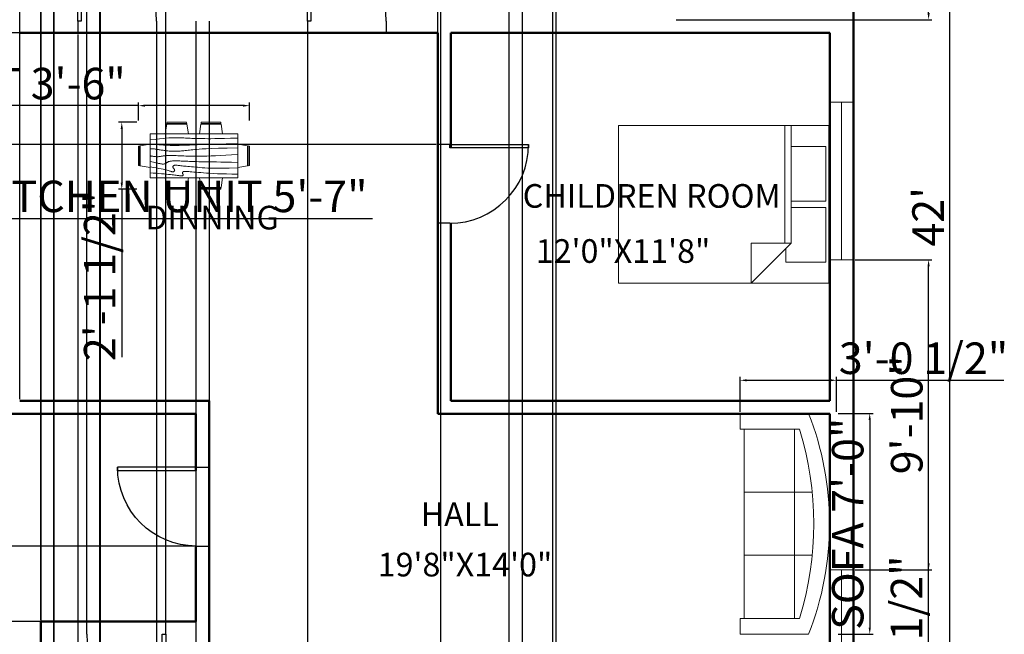
# Model space of a CAD drawing. Units: inches. Extents: x 2744 to 3775, y 2156 to 2963.
# Tile 3 of 4: x 3167 to 3541, y 2346 to 2580. Entities that reach past the tile are written whole.
import ezdxf

# ---------------------------------------------------------------- set-up
doc = ezdxf.new("R2010")
doc.units = ezdxf.units.IN
for name, color, linetype, lineweight in [('A-ANNO-DIMS', 2, 'Continuous', 18), ('A-AREA-IDEN', 7, 'Continuous', 25), ('A-DOOR', 3, 'Continuous', 25), ('A-FURN', 8, 'Continuous', 18), ('A-GLAZ', 4, 'Continuous', 18), ('A-WALL', 7, 'Continuous', 50)]:
    doc.layers.add(name, color=color, linetype=linetype, lineweight=lineweight)
doc.styles.get("Standard").update_dxf_attribs({"font": 'arial.ttf'})
doc.dimstyles.new('ISO-25', dxfattribs={"dimtxt": 12, "dimasz": 2.5, "dimexe": 1.25, "dimexo": 0.625, "dimtad": 1, "dimdec": 1, "dimlunit": 4, "dimtxsty": 'Standard', "dimcen": 2.5, "dimadec": 0, "dimazin": 0, "dimtfac": 1, "dimtdec": 1, "dimtmove": 0, "dimatfit": 3, "dimfxl": 1, "dimarcsym": 0})

# ---------------------------------------------------------------- blocks, each defined once
blk = doc.blocks.new('*U2')
for p, q in [((0, 0), (0, -6)), ((40, 0), (40, -6))]:
    blk.add_line(p, q)
blk.add_lwpolyline([(0, 0), (0, 40), (1.75, 40), (1.75, 0)], close=True)
blk.add_arc((0, 0), 40, 0, 90)
blk = doc.blocks.new('Bed - Queen')
for p, q in [((0, -80.00003), (0, 0)), ((0, 0), (59.99999, 0)), ((59.99999, 0), (59.99999, -80.00003)), ((7.99999, -1.2), (28.79998, -1.2)), ((7.99999, -14.4), (7.99999, -1.2)), ((28.79998, -1.2), (28.79998, -14.4)), ((31.19999, -1.2), (51.99999, -1.2)), ((31.19999, -14.4), (31.19999, -1.2)), ((51.99999, -1.2), (51.99999, -16.4)), ((0, -14.4), (44.8, -14.4)), ((59.99999, -29.6), (44.8, -14.4)), ((44.8, -14.4), (44.8, -29.6)), ((44.8, -16.8), (0, -16.8)), ((51.99999, -16.4), (46.79936, -16.4)), ((44.8, -29.6), (59.99999, -29.6)), ((59.99999, -80.00003), (0, -80.00003))]:
    blk.add_line(p, q)
blk = doc.blocks.new('Sofa - Roundback 7 ft.')
for p, q in [((-12.00002, -32.4421), (-12.00003, -6.5971)), ((11.99997, -32.4421), (11.99998, -6.5971)), ((-36.000027, -34), (-36.000027, -11.4696)), ((-35.999844, -13.3819), (35.9998, -13.3819)), ((35.99998, -34), (35.99998, -11.4696)), ((-36.000027, -32.4421), (35.99998, -32.4421))]:
    blk.add_line(p, q)
for points in [[(-36.000027, -34), (-42.000027, -34), (-42.000027, -8)], [(41.99998, -8), (41.99998, -34), (35.99998, -34)]]:
    blk.add_lwpolyline(points)
for centre, radius, start, end in [((0, -114.25), 114.25, 68.43141, 111.5686), ((-0.00001, -127.1968), 121.1968, 72.72033, 107.2797)]:
    blk.add_arc(centre, radius, start, end)
blk = doc.blocks.new('Dining Set - 36 x 72 in.')
for p, q in [((-22.2343, 26.00059), (-23.4847, 17.99762)), ((-22.2304, 26), (-5.7608, 26)), ((-22, 27.5), (-22.1562, 26.50042)), ((-5.8416, 26.5), (-22.1534, 26.5)), ((-22, 27.5), (-6, 27.5)), ((-5.8437, 26.49966), (-6, 27.5)), ((-4.5152, 17.99762), (-5.7655, 25.99926)), ((5.7657, 26.00059), (4.5153, 17.99762)), ((5.7696, 26), (22.2392, 26)), ((6, 27.5), (5.8438, 26.50042)), ((22.1584, 26.5), (5.8466, 26.5)), ((6, 27.5), (22, 27.5)), ((22.1563, 26.49966), (22, 27.5)), ((23.4848, 17.99762), (22.2345, 25.99926)), ((36, 18), (-36, 18)), ((-36, 18), (-36, -18)), ((36, -18), (36, 18)), ((-45.5, 8), (-44.5004, 8.15617)), ((-44.5, -8.15843), (-44.5, 8.15338)), ((-44.0006, 8.23428), (-35.9976, 9.48474)), ((-44, 8.23041), (-44, -8.23915)), ((44.0006, 8.23428), (35.9976, 9.48474)), ((44, 8.23041), (44, -8.23915)), ((44.5, -8.15843), (44.5, 8.15338)), ((45.5, 8), (44.5005, 8.15617)), ((-45.5, 8), (-45.5, -8)), ((45.5, 8), (45.5, -8)), ((-44.4997, -8.15631), (-45.5, -8)), ((44.4997, -8.15631), (45.5, -8)), ((-35.9976, -9.48476), (-43.9993, -8.2345)), ((35.9976, -9.48476), (43.9993, -8.2345)), ((-36, -18), (36, -18)), ((-22.2343, -26.0006), (-23.4847, -17.99762)), ((-4.5152, -17.99762), (-5.7655, -25.99928)), ((5.7657, -26.0006), (4.5153, -17.99762)), ((23.4848, -17.99762), (22.2345, -25.99928)), ((-22.2304, -26), (-5.7608, -26)), ((-22, -27.5), (-22.1562, -26.50044)), ((-5.8416, -26.5), (-22.1534, -26.5)), ((-22, -27.5), (-6, -27.5)), ((-5.8437, -26.49967), (-6, -27.5)), ((5.7696, -26), (22.2392, -26)), ((6, -27.5), (5.8438, -26.50044)), ((22.1584, -26.5), (5.8466, -26.5)), ((6, -27.5), (22, -27.5)), ((22.1563, -26.49967), (22, -27.5))]:
    blk.add_line(p, q)
for points in [[(-36, 15), (-31.1772, 14.97754), (-26.8079, 14.91406), (-22.8538, 14.81543), (-19.276, 14.6875), (-16.0362, 14.53613), (-13.0957, 14.36718), (-10.4159, 14.18652), (-7.9583, 14), (-5.6904, 13.81315), (-3.6035, 13.63021), (-1.6954, 13.45508), (0.0365, 13.29166), (1.5945, 13.14388), (2.9811, 13.01562), (4.1988, 12.9108), (5.25, 12.83333), (6.1393, 12.78613), (6.8802, 12.76823), (7.4883, 12.77767), (7.9792, 12.8125), (8.3685, 12.87077), (8.6719, 12.95052), (8.9049, 13.0498), (9.0833, 13.16666), (9.2205, 13.29899), (9.3216, 13.44401), (9.3895, 13.59879), (9.4271, 13.76041), (9.4373, 13.92594), (9.4232, 14.09245), (9.3875, 14.257), (9.3333, 14.41666), (9.2638, 14.56917), (9.1836, 14.71484), (9.0975, 14.85465), (9.0104, 14.98958), (8.9272, 15.1206), (8.8529, 15.2487), (8.7922, 15.37483), (8.75, 15.5), (8.7305, 15.62467), (8.7344, 15.74739), (8.7617, 15.86621), (8.8125, 15.97916), (8.8867, 16.08431), (8.9844, 16.17968), (9.1055, 16.26334), (9.25, 16.33333), (9.4189, 16.38802), (9.6172, 16.42708), (9.8506, 16.45052), (10.125, 16.45833), (10.4463, 16.45052), (10.8203, 16.42708), (11.2529, 16.38802), (11.75, 16.33333), (12.3184, 16.26318), (12.9694, 16.17838), (13.7151, 16.07991), (14.5677, 15.96875), (15.5395, 15.84586), (16.6426, 15.71224), (17.8893, 15.56884), (19.2917, 15.41666), (20.859, 15.25667), (22.5879, 15.08984), (24.4721, 14.91715), (26.5052, 14.73958), (28.6809, 14.5581), (30.9929, 14.3737), (33.4347, 14.18733), (36, 14)], [(-36, 10), (-28.9766, 10.14274), (-23.1725, 10.20442), (-18.4241, 10.19775), (-14.5677, 10.13541), (-11.4399, 10.03011), (-8.877, 9.89453), (-6.7154, 9.74137), (-4.7917, 9.58333), (-2.9698, 9.43082), (-1.2246, 9.28515), (0.4415, 9.14534), (2.026, 9.01041), (3.5266, 8.87939), (4.9408, 8.7513), (6.266, 8.62516), (7.5, 8.5), (8.6411, 8.37549), (9.6914, 8.2539), (10.6538, 8.13818), (11.5312, 8.03125), (12.3267, 7.93603), (13.043, 7.85547), (13.6831, 7.79248), (14.25, 7.75), (14.7471, 7.7303), (15.1797, 7.73307), (15.5537, 7.75732), (15.875, 7.80208), (16.1494, 7.86637), (16.3828, 7.94922), (16.5811, 8.04964), (16.75, 8.16666), (16.8944, 8.29915), (17.0143, 8.44531), (17.1089, 8.60319), (17.1771, 8.77083), (17.218, 8.94629), (17.2305, 9.1276), (17.2137, 9.31282), (17.1667, 9.5), (17.0895, 9.6875), (16.987, 9.875), (16.8649, 10.0625), (16.7292, 10.25), (16.5856, 10.4375), (16.4401, 10.625), (16.2985, 10.8125), (16.1667, 11), (16.05, 11.18733), (15.9518, 11.3737), (15.8752, 11.5581), (15.8229, 11.73958), (15.798, 11.91715), (15.8034, 12.08984), (15.842, 12.25667), (15.9167, 12.41666), (16.0295, 12.56836), (16.1784, 12.70833), (16.3605, 12.83268), (16.5729, 12.9375), (16.8127, 13.01888), (17.0768, 13.07291), (17.3625, 13.0957), (17.6667, 13.08333), (17.9894, 13.03312), (18.3418, 12.94726), (18.7382, 12.82918), (19.1927, 12.68229), (19.7195, 12.51001), (20.3327, 12.31575), (21.0465, 12.10294), (21.875, 11.875), (22.8357, 11.63354), (23.959, 11.37304), (25.2786, 11.08618), (26.8282, 10.76562), (28.6414, 10.40405), (30.752, 9.99414), (33.1936, 9.52856), (36, 9)], [(-36, 5.5), (-30.7157, 5.3348), (-26.069, 5.20963), (-21.9946, 5.11767), (-18.4271, 5.05208), (-15.3009, 5.00602), (-12.5508, 4.97265), (-10.1112, 4.94515), (-7.9167, 4.91666), (-5.909, 4.88167), (-4.0586, 4.83984), (-2.3429, 4.79215), (-0.7396, 4.73958), (0.7739, 4.6831), (2.22, 4.6237), (3.6213, 4.56233), (5, 4.5), (6.373, 4.43782), (7.7344, 4.3776), (9.0723, 4.32129), (10.375, 4.27083), (11.6309, 4.22819), (12.8281, 4.19531), (13.9551, 4.17415), (15, 4.16666), (15.954, 4.17448), (16.819, 4.19791), (17.6001, 4.23698), (18.3021, 4.29166), (18.9299, 4.36198), (19.4883, 4.44791), (19.9823, 4.54948), (20.4167, 4.66666), (20.7969, 4.79899), (21.1302, 4.94401), (21.4245, 5.09879), (21.6875, 5.26041), (21.9271, 5.42594), (22.1511, 5.59245), (22.3672, 5.757), (22.5834, 5.91666), (22.8065, 6.06868), (23.0404, 6.21093), (23.2879, 6.34147), (23.5521, 6.45833), (23.8358, 6.55957), (24.142, 6.64323), (24.4735, 6.70735), (24.8334, 6.75), (25.2235, 6.76969), (25.642, 6.76692), (26.0858, 6.74267), (26.5521, 6.69791), (27.0379, 6.63362), (27.5404, 6.55078), (28.0565, 6.45036), (28.5834, 6.33333), (29.1242, 6.19987), (29.7071, 6.04687), (30.3661, 5.87044), (31.1354, 5.66666), (32.0493, 5.43164), (33.142, 5.16146), (34.4475, 4.85221), (36, 4.5)], [(-36, -1), (-30.7915, -0.6591), (-26.0195, -0.38216), (-21.6519, -0.16284), (-17.6563, 0.00521), (-14.0005, 0.12833), (-10.6523, 0.21289), (-7.5796, 0.26522), (-4.75, 0.29166), (-2.134, 0.29793), (0.2878, 0.28711), (2.5317, 0.26163), (4.6146, 0.22396), (6.5529, 0.17651), (8.3633, 0.12174), (10.0623, 0.06209), (11.6667, 0), (13.1899, -0.06201), (14.6341, -0.1211), (15.9982, -0.17432), (17.2813, -0.21875), (18.4823, -0.25147), (19.6003, -0.26953), (20.6343, -0.27002), (21.5834, -0.25), (22.4481, -0.20768), (23.2357, -0.14584), (23.9549, -0.06836), (24.6146, 0.02083), (25.2235, 0.11784), (25.7904, 0.21875), (26.3241, 0.31966), (26.8334, 0.41666), (27.3265, 0.50618), (27.8099, 0.58593), (28.2894, 0.65397), (28.7709, 0.70833), (29.2601, 0.74707), (29.763, 0.76823), (30.2855, 0.76985), (30.8334, 0.75), (31.4088, 0.70784), (31.9994, 0.64713), (32.589, 0.57275), (33.1615, 0.48958), (33.7008, 0.4025), (34.1908, 0.3164), (34.6153, 0.23616), (34.9584, 0.16666), (35.2099, 0.11165), (35.3848, 0.07031), (35.504, 0.04069), (35.5886, 0.02083), (35.6594, 0.00879), (35.7377, 0.0026), (35.8442, 0.00032), (36, 0)], [(-36, -6.5), (-27.1843, -6.31267), (-20.084, -6.1263), (-14.469, -5.9419), (-10.1094, -5.76042), (-6.7752, -5.58285), (-4.2363, -5.41016), (-2.2629, -5.24333), (-0.625, -5.08334), (0.8708, -4.93099), (2.2715, -4.78646), (3.5872, -4.64974), (4.8281, -4.52084), (6.0046, -4.39974), (7.127, -4.28646), (8.2053, -4.18099), (9.25, -4.08334), (10.2705, -3.99382), (11.2734, -3.91407), (12.2647, -3.84603), (13.25, -3.79167), (14.2354, -3.75293), (15.2266, -3.73177), (16.2295, -3.73015), (17.25, -3.75), (18.2912, -3.79248), (19.3451, -3.85547), (20.4009, -3.93604), (21.4479, -4.03125), (22.4754, -4.13819), (23.4727, -4.25391), (24.4289, -4.37549), (25.3334, -4.5), (26.1785, -4.62492), (26.9694, -4.74935), (27.7145, -4.87281), (28.4219, -4.99479), (29.1, -5.11483), (29.7572, -5.23242), (30.4016, -5.34709), (31.0417, -5.45834), (31.6837, -5.56437), (32.3262, -5.65821), (32.9658, -5.73153), (33.599, -5.77604), (34.2224, -5.78345), (34.8327, -5.74545), (35.4264, -5.65373), (36, -5.5)], [(-36, -10), (-26.4022, -9.81299), (-18.4675, -9.62891), (-11.9839, -9.45069), (-6.7396, -9.28125), (-2.5226, -9.12354), (0.8789, -8.98047), (3.6769, -8.85498), (6.0833, -8.75), (8.2767, -8.66765), (10.3021, -8.60677), (12.1712, -8.56543), (13.8958, -8.54167), (15.4876, -8.53353), (16.9583, -8.53907), (18.3197, -8.55632), (19.5834, -8.58334), (20.7616, -8.61841), (21.8685, -8.66081), (22.9188, -8.71004), (23.9271, -8.76563), (24.9081, -8.82707), (25.8763, -8.89388), (26.8465, -8.96558), (27.8334, -9.04167), (28.8474, -9.12118), (29.8828, -9.20117), (30.93, -9.27824), (31.9792, -9.34896), (33.0205, -9.40991), (34.0443, -9.45768), (35.0407, -9.48885), (36, -9.5)], [(-36, -14.5), (-30.0881, -14.33513), (-25.0332, -14.21224), (-20.7312, -14.12647), (-17.0781, -14.07292), (-13.97, -14.04671), (-11.3027, -14.04297), (-8.9724, -14.05681), (-6.875, -14.08334), (-4.9224, -14.11833), (-3.0905, -14.16016), (-1.3709, -14.20785), (0.2448, -14.26042), (1.7647, -14.3169), (3.1973, -14.3763), (4.5507, -14.43767), (5.8333, -14.5), (7.0554, -14.5621), (8.235, -14.62175), (9.3922, -14.67652), (10.5469, -14.72396), (11.7192, -14.76164), (12.929, -14.78711), (14.1965, -14.79794), (15.5417, -14.79167), (16.9933, -14.76424), (18.6152, -14.70508), (20.4804, -14.60197), (22.6615, -14.44271), (25.2312, -14.21509), (28.2624, -13.9069), (31.8277, -13.50594), (36, -13)]]:
    blk.add_lwpolyline(points)
blk = doc.blocks.new('*D15')
at = {"layer": 'A-ANNO-DIMS', "color": 0, "lineweight": -2, "transparency": 16777216}
for p, q in [((3484.55, 2757.1), (3521.77, 2757.1)), ((3520.52, 2754.6), (3520.52, 2255.6)), ((3484.55, 2253.1), (3521.77, 2253.1))]:
    blk.add_line(p, q, dxfattribs=at)
at = {"layer": 'A-ANNO-DIMS', "color": 0, "transparency": 16777216}
for points in [[(3520.11, 2754.6), (3520.94, 2754.6), (3520.52, 2757.1)], [(3520.11, 2255.6), (3520.94, 2255.6), (3520.52, 2253.1)]]:
    blk.add_solid(points, dxfattribs=at)
at = {"layer": 'Defpoints', "color": 0, "transparency": 16777216}
for p in [(3483.92, 2757.1), (3483.92, 2253.1), (3520.52, 2253.1)]:
    blk.add_point(p, dxfattribs=at)
at = {"layer": 'A-ANNO-DIMS', "color": 0, "transparency": 16777216, "insert": (3513.88, 2505.1), "char_height": 12, "attachment_point": 5, "rotation": 90}
blk.add_mtext("42'", dxfattribs=at)
blk = doc.blocks.new('WIN-60IN')
blk.add_line((0, 4.5), (60, 4.5))
blk.add_lwpolyline([(0, 9), (60, 9), (60, 0), (0, 0)], close=True)
blk = doc.blocks.new('*D26')
at = {"layer": 'A-ANNO-DIMS', "color": 0, "lineweight": -2, "transparency": 16777216}
for p, q in [((3478.16, 2430.27), (3491.39, 2430.27)), ((3490.14, 2427.77), (3490.14, 2348.77)), ((3478.16, 2346.27), (3491.39, 2346.27))]:
    blk.add_line(p, q, dxfattribs=at)
at = {"layer": 'A-ANNO-DIMS', "color": 0, "transparency": 16777216}
for points in [[(3489.72, 2427.77), (3490.56, 2427.77), (3490.14, 2430.27)], [(3489.72, 2348.77), (3490.56, 2348.77), (3490.14, 2346.27)]]:
    blk.add_solid(points, dxfattribs=at)
at = {"layer": 'Defpoints', "color": 0, "transparency": 16777216}
for p in [(3477.54, 2430.27), (3477.54, 2346.27), (3490.14, 2346.27)]:
    blk.add_point(p, dxfattribs=at)
at = {"layer": 'A-ANNO-DIMS', "color": 0, "transparency": 16777216, "insert": (3483.31, 2388.27), "char_height": 12, "attachment_point": 5, "rotation": 90}
blk.add_mtext('SOFA 7\'-0"', dxfattribs=at)
blk = doc.blocks.new('*D27')
at = {"layer": 'A-ANNO-DIMS', "color": 0, "lineweight": -2, "transparency": 16777216}
for p, q in [((3440.87, 2430.89), (3440.87, 2444.12)), ((3443.37, 2442.87), (3475.04, 2442.87)), ((3477.54, 2430.89), (3477.54, 2444.12)), ((3477.54, 2442.87), (3541.14, 2442.87))]:
    blk.add_line(p, q, dxfattribs=at)
at = {"layer": 'A-ANNO-DIMS', "color": 0, "transparency": 16777216}
for points in [[(3443.37, 2443.28), (3443.37, 2442.45), (3440.87, 2442.87)], [(3475.04, 2443.28), (3475.04, 2442.45), (3477.54, 2442.87)]]:
    blk.add_solid(points, dxfattribs=at)
at = {"layer": 'Defpoints', "color": 0, "transparency": 16777216}
for p in [(3477.54, 2442.87), (3440.87, 2430.27), (3477.54, 2430.27)]:
    blk.add_point(p, dxfattribs=at)
at = {"layer": 'A-ANNO-DIMS', "color": 0, "transparency": 16777216, "insert": (3510.59, 2449.7), "char_height": 12, "attachment_point": 5}
blk.add_mtext('3\'-0 1/2"', dxfattribs=at)
blk = doc.blocks.new('*D30')
at = {"layer": 'A-ANNO-DIMS', "color": 0, "lineweight": -2, "transparency": 16777216}
for p, q in [((3077.09, 2495.06), (3077.09, 2505.72)), ((3143.99, 2495.06), (3143.99, 2505.72)), ((3079.59, 2504.47), (3141.49, 2504.47)), ((3143.99, 2504.47), (3301.12, 2504.47))]:
    blk.add_line(p, q, dxfattribs=at)
at = {"layer": 'A-ANNO-DIMS', "color": 0, "transparency": 16777216}
for points in [[(3079.59, 2504.89), (3079.59, 2504.06), (3077.09, 2504.47)], [(3141.49, 2504.89), (3141.49, 2504.06), (3143.99, 2504.47)]]:
    blk.add_solid(points, dxfattribs=at)
at = {"layer": 'Defpoints', "color": 0, "transparency": 16777216}
for p in [(3143.99, 2504.47), (3077.09, 2494.44), (3143.99, 2494.44)]:
    blk.add_point(p, dxfattribs=at)
at = {"layer": 'A-ANNO-DIMS', "color": 0, "transparency": 16777216, "insert": (3223.81, 2511.3), "char_height": 12, "attachment_point": 5}
blk.add_mtext('KITCHEN UNIT 5\'-7"', dxfattribs=at)
blk = doc.blocks.new('*D32')
at = {"layer": 'A-ANNO-DIMS', "color": 0, "lineweight": -2, "transparency": 16777216}
for p, q in [((3212.07, 2547.39), (3076.42, 2547.39)), ((3212.07, 2541.68), (3212.07, 2548.64)), ((3251.79, 2547.39), (3214.57, 2547.39)), ((3254.29, 2541.68), (3254.29, 2548.64))]:
    blk.add_line(p, q, dxfattribs=at)
at = {"layer": 'A-ANNO-DIMS', "color": 0, "transparency": 16777216}
for points in [[(3214.57, 2547.81), (3214.57, 2546.97), (3212.07, 2547.39)], [(3251.79, 2547.81), (3251.79, 2546.97), (3254.29, 2547.39)]]:
    blk.add_solid(points, dxfattribs=at)
at = {"layer": 'Defpoints', "color": 0, "transparency": 16777216}
for p in [(3212.07, 2547.39), (3212.07, 2541.06), (3254.29, 2541.06)]:
    blk.add_point(p, dxfattribs=at)
at = {"layer": 'A-ANNO-DIMS', "color": 0, "transparency": 16777216, "insert": (3143, 2554.22), "char_height": 12, "attachment_point": 5}
blk.add_mtext('DINING SET 3\'-6"', dxfattribs=at)
blk = doc.blocks.new('*D33')
at = {"layer": 'A-ANNO-DIMS', "color": 0, "lineweight": -2, "transparency": 16777216}
for p, q in [((3211.44, 2541.06), (3204.48, 2541.06)), ((3205.73, 2538.56), (3205.73, 2518.04)), ((3211.44, 2515.54), (3204.48, 2515.54)), ((3205.73, 2515.54), (3205.73, 2451.72))]:
    blk.add_line(p, q, dxfattribs=at)
at = {"layer": 'A-ANNO-DIMS', "color": 0, "transparency": 16777216}
for points in [[(3205.32, 2538.56), (3206.15, 2538.56), (3205.73, 2541.06)], [(3205.32, 2518.04), (3206.15, 2518.04), (3205.73, 2515.54)]]:
    blk.add_solid(points, dxfattribs=at)
at = {"layer": 'Defpoints', "color": 0, "transparency": 16777216}
for p in [(3212.07, 2541.06), (3205.73, 2515.54), (3212.07, 2515.54)]:
    blk.add_point(p, dxfattribs=at)
at = {"layer": 'A-ANNO-DIMS', "color": 0, "transparency": 16777216, "insert": (3198.9, 2482.38), "char_height": 12, "attachment_point": 5, "rotation": 90}
blk.add_mtext('2\'-1 1/2"', dxfattribs=at)
blk = doc.blocks.new('*D34')
at = {"layer": 'A-ANNO-DIMS', "color": 0, "lineweight": -2, "transparency": 16777216}
for p, q in [((3145.86, 2747.48), (3145.86, 2223.25)), ((3174.92, 2747.48), (3174.92, 2223.25)), ((3148.36, 2224.5), (3172.42, 2224.5)), ((3174.92, 2224.5), (3210.78, 2224.5))]:
    blk.add_line(p, q, dxfattribs=at)
at = {"layer": 'A-ANNO-DIMS', "color": 0, "transparency": 16777216}
for points in [[(3148.36, 2224.92), (3148.36, 2224.09), (3145.86, 2224.5)], [(3172.42, 2224.92), (3172.42, 2224.09), (3174.92, 2224.5)]]:
    blk.add_solid(points, dxfattribs=at)
at = {"layer": 'Defpoints', "color": 0, "transparency": 16777216}
for p in [(3145.86, 2748.1), (3174.92, 2748.1), (3174.92, 2224.5)]:
    blk.add_point(p, dxfattribs=at)
at = {"layer": 'A-ANNO-DIMS', "color": 0, "transparency": 16777216, "insert": (3194.1, 2231.26), "char_height": 12, "attachment_point": 5}
blk.add_mtext('2\'-5"', dxfattribs=at)
blk = doc.blocks.new('*D35')
at = {"layer": 'A-ANNO-DIMS', "color": 0, "lineweight": -2, "transparency": 16777216}
for p, q in [((3179.92, 2747.48), (3179.92, 2223.25)), ((3197.52, 2747.48), (3197.52, 2223.25)), ((3182.42, 2224.5), (3195.02, 2224.5)), ((3197.52, 2224.5), (3260.01, 2224.5))]:
    blk.add_line(p, q, dxfattribs=at)
at = {"layer": 'A-ANNO-DIMS', "color": 0, "transparency": 16777216}
for points in [[(3182.42, 2224.92), (3182.42, 2224.09), (3179.92, 2224.5)], [(3195.02, 2224.92), (3195.02, 2224.09), (3197.52, 2224.5)]]:
    blk.add_solid(points, dxfattribs=at)
at = {"layer": 'Defpoints', "color": 0, "transparency": 16777216}
for p in [(3179.92, 2748.1), (3197.52, 2748.1), (3197.52, 2224.5)]:
    blk.add_point(p, dxfattribs=at)
at = {"layer": 'A-ANNO-DIMS', "color": 0, "transparency": 16777216, "insert": (3230.02, 2231.33), "char_height": 12, "attachment_point": 5}
blk.add_mtext('1\'-5 1/2"', dxfattribs=at)
blk = doc.blocks.new('*D36')
at = {"layer": 'A-ANNO-DIMS', "color": 0, "lineweight": -2, "transparency": 16777216}
for p, q in [((3326.88, 2747.48), (3326.88, 2223.25)), ((3352.92, 2747.48), (3352.92, 2223.25)), ((3329.38, 2224.5), (3350.42, 2224.5)), ((3352.92, 2224.5), (3388.78, 2224.5))]:
    blk.add_line(p, q, dxfattribs=at)
at = {"layer": 'A-ANNO-DIMS', "color": 0, "transparency": 16777216}
for points in [[(3329.38, 2224.92), (3329.38, 2224.09), (3326.88, 2224.5)], [(3350.42, 2224.92), (3350.42, 2224.09), (3352.92, 2224.5)]]:
    blk.add_solid(points, dxfattribs=at)
at = {"layer": 'Defpoints', "color": 0, "transparency": 16777216}
for p in [(3326.88, 2748.1), (3352.92, 2748.1), (3352.92, 2224.5)]:
    blk.add_point(p, dxfattribs=at)
at = {"layer": 'A-ANNO-DIMS', "color": 0, "transparency": 16777216, "insert": (3372.1, 2231.15), "char_height": 12, "attachment_point": 5}
blk.add_mtext('2\'-2"', dxfattribs=at)
blk = doc.blocks.new('*D37')
at = {"layer": 'A-ANNO-DIMS', "color": 0, "lineweight": -2, "transparency": 16777216}
for p, q in [((3357.92, 2747.48), (3357.92, 2223.25)), ((3370.78, 2747.48), (3370.78, 2223.25)), ((3360.42, 2224.5), (3368.28, 2224.5)), ((3370.78, 2224.5), (3405.3, 2224.5))]:
    blk.add_line(p, q, dxfattribs=at)
at = {"layer": 'A-ANNO-DIMS', "color": 0, "transparency": 16777216}
for points in [[(3360.42, 2224.92), (3360.42, 2224.09), (3357.92, 2224.5)], [(3368.28, 2224.92), (3368.28, 2224.09), (3370.78, 2224.5)]]:
    blk.add_solid(points, dxfattribs=at)
at = {"layer": 'Defpoints', "color": 0, "transparency": 16777216}
for p in [(3357.92, 2748.1), (3370.78, 2748.1), (3370.78, 2224.5)]:
    blk.add_point(p, dxfattribs=at)
at = {"layer": 'A-ANNO-DIMS', "color": 0, "transparency": 16777216, "insert": (3389.29, 2231.15), "char_height": 12, "attachment_point": 5}
blk.add_mtext('1\'-1"', dxfattribs=at)
blk = doc.blocks.new('*D39')
at = {"layer": 'A-ANNO-DIMS', "color": 0, "lineweight": -2, "transparency": 16777216}
for p, q in [((3179.92, 2262.73), (3179.92, 2786.95)), ((3182.42, 2785.7), (3194.86, 2785.7)), ((3197.36, 2262.73), (3197.36, 2786.95)), ((3197.36, 2785.7), (3259.85, 2785.7))]:
    blk.add_line(p, q, dxfattribs=at)
at = {"layer": 'A-ANNO-DIMS', "color": 0, "transparency": 16777216}
for points in [[(3182.42, 2786.12), (3182.42, 2785.29), (3179.92, 2785.7)], [(3194.86, 2786.12), (3194.86, 2785.29), (3197.36, 2785.7)]]:
    blk.add_solid(points, dxfattribs=at)
at = {"layer": 'Defpoints', "color": 0, "transparency": 16777216}
for p in [(3197.36, 2785.7), (3179.92, 2262.1), (3197.36, 2262.1)]:
    blk.add_point(p, dxfattribs=at)
at = {"layer": 'A-ANNO-DIMS', "color": 0, "transparency": 16777216, "insert": (3229.85, 2792.53), "char_height": 12, "attachment_point": 5}
blk.add_mtext('1\'-5 1/2"', dxfattribs=at)
blk = doc.blocks.new('*D43')
at = {"layer": 'A-ANNO-DIMS', "color": 0, "lineweight": -2, "transparency": 16777216}
for p, q in [((3512.52, 2310.69), (3512.52, 2374.78)), ((3484.55, 2310.69), (3513.77, 2310.69)), ((3512.52, 2255.6), (3512.52, 2308.19)), ((3484.55, 2253.1), (3513.77, 2253.1))]:
    blk.add_line(p, q, dxfattribs=at)
at = {"layer": 'A-ANNO-DIMS', "color": 0, "transparency": 16777216}
for points in [[(3512.11, 2308.19), (3512.94, 2308.19), (3512.52, 2310.69)], [(3512.11, 2255.6), (3512.94, 2255.6), (3512.52, 2253.1)]]:
    blk.add_solid(points, dxfattribs=at)
at = {"layer": 'Defpoints', "color": 0, "transparency": 16777216}
for p in [(3483.92, 2310.69), (3512.52, 2310.69), (3483.92, 2253.1)]:
    blk.add_point(p, dxfattribs=at)
at = {"layer": 'A-ANNO-DIMS', "color": 0, "transparency": 16777216, "insert": (3505.69, 2343.99), "char_height": 12, "attachment_point": 5, "rotation": 90}
blk.add_mtext('4\'-9 1/2"', dxfattribs=at)
blk = doc.blocks.new('*D44')
at = {"layer": 'A-ANNO-DIMS', "color": 0, "lineweight": -2, "transparency": 16777216}
for p, q in [((3484.55, 2488.72), (3513.77, 2488.72)), ((3512.52, 2373.19), (3512.52, 2486.22)), ((3484.55, 2370.69), (3513.77, 2370.69))]:
    blk.add_line(p, q, dxfattribs=at)
at = {"layer": 'A-ANNO-DIMS', "color": 0, "transparency": 16777216}
for points in [[(3512.11, 2486.22), (3512.94, 2486.22), (3512.52, 2488.72)], [(3512.11, 2373.19), (3512.94, 2373.19), (3512.52, 2370.69)]]:
    blk.add_solid(points, dxfattribs=at)
at = {"layer": 'Defpoints', "color": 0, "transparency": 16777216}
for p in [(3483.92, 2488.72), (3512.52, 2488.72), (3483.92, 2370.69)]:
    blk.add_point(p, dxfattribs=at)
at = {"layer": 'A-ANNO-DIMS', "color": 0, "transparency": 16777216, "insert": (3505.77, 2429.71), "char_height": 12, "attachment_point": 5, "rotation": 90}
blk.add_mtext('9\'-10"', dxfattribs=at)
blk = doc.blocks.new('*D45')
at = {"layer": 'A-ANNO-DIMS', "color": 0, "lineweight": -2, "transparency": 16777216}
for p, q in [((3188.98, 2574.48), (3188.98, 2223.25)), ((3218.98, 2574.48), (3218.98, 2223.25)), ((3191.48, 2224.5), (3216.48, 2224.5)), ((3218.98, 2224.5), (3254.83, 2224.5))]:
    blk.add_line(p, q, dxfattribs=at)
at = {"layer": 'A-ANNO-DIMS', "color": 0, "transparency": 16777216}
for points in [[(3191.48, 2224.92), (3191.48, 2224.09), (3188.98, 2224.5)], [(3216.48, 2224.92), (3216.48, 2224.09), (3218.98, 2224.5)]]:
    blk.add_solid(points, dxfattribs=at)
at = {"layer": 'Defpoints', "color": 0, "transparency": 16777216}
for p in [(3188.98, 2575.1), (3218.98, 2575.1), (3218.98, 2224.5)]:
    blk.add_point(p, dxfattribs=at)
at = {"layer": 'A-ANNO-DIMS', "color": 0, "transparency": 16777216, "insert": (3238.16, 2231.26), "char_height": 12, "attachment_point": 5}
blk.add_mtext('2\'-6"', dxfattribs=at)
blk = doc.blocks.new('*D46')
at = {"layer": 'A-ANNO-DIMS', "color": 0, "lineweight": -2, "transparency": 16777216}
for p, q in [((3218.97, 2579.48), (3218.97, 2223.25)), ((3233.92, 2579.48), (3233.92, 2223.25)), ((3221.47, 2224.5), (3231.42, 2224.5)), ((3233.92, 2224.5), (3268.44, 2224.5))]:
    blk.add_line(p, q, dxfattribs=at)
at = {"layer": 'A-ANNO-DIMS', "color": 0, "transparency": 16777216}
for points in [[(3221.47, 2224.92), (3221.47, 2224.09), (3218.97, 2224.5)], [(3231.42, 2224.92), (3231.42, 2224.09), (3233.92, 2224.5)]]:
    blk.add_solid(points, dxfattribs=at)
at = {"layer": 'Defpoints', "color": 0, "transparency": 16777216}
for p in [(3218.97, 2580.1), (3233.92, 2580.1), (3233.92, 2224.5)]:
    blk.add_point(p, dxfattribs=at)
at = {"layer": 'A-ANNO-DIMS', "color": 0, "transparency": 16777216, "insert": (3252.43, 2231.26), "char_height": 12, "attachment_point": 5}
blk.add_mtext('1\'-3"', dxfattribs=at)
blk = doc.blocks.new('*D47')
at = {"layer": 'A-ANNO-DIMS', "color": 0, "lineweight": -2, "transparency": 16777216}
for p, q in [((3238.92, 2579.48), (3238.92, 2223.25)), ((3276.3, 2578.98), (3276.3, 2223.25)), ((3241.42, 2224.5), (3273.8, 2224.5)), ((3276.3, 2224.5), (3339.9, 2224.5))]:
    blk.add_line(p, q, dxfattribs=at)
at = {"layer": 'A-ANNO-DIMS', "color": 0, "transparency": 16777216}
for points in [[(3241.42, 2224.92), (3241.42, 2224.09), (3238.92, 2224.5)], [(3273.8, 2224.92), (3273.8, 2224.09), (3276.3, 2224.5)]]:
    blk.add_solid(points, dxfattribs=at)
at = {"layer": 'Defpoints', "color": 0, "transparency": 16777216}
for p in [(3238.92, 2580.1), (3276.3, 2579.6), (3276.3, 2224.5)]:
    blk.add_point(p, dxfattribs=at)
at = {"layer": 'A-ANNO-DIMS', "color": 0, "transparency": 16777216, "insert": (3309.35, 2231.34), "char_height": 12, "attachment_point": 5}
blk.add_mtext('3\'-1 1/2"', dxfattribs=at)
blk = doc.blocks.new('*D52')
at = {"layer": 'A-ANNO-DIMS', "color": 0, "lineweight": -2, "transparency": 16777216}
for p, q in [((3166.92, 2435.73), (3166.92, 2786.95)), ((3169.42, 2785.7), (3323.42, 2785.7)), ((3325.92, 2430.73), (3325.92, 2786.95))]:
    blk.add_line(p, q, dxfattribs=at)
at = {"layer": 'A-ANNO-DIMS', "color": 0, "transparency": 16777216}
for points in [[(3169.42, 2786.12), (3169.42, 2785.29), (3166.92, 2785.7)], [(3323.42, 2786.12), (3323.42, 2785.29), (3325.92, 2785.7)]]:
    blk.add_solid(points, dxfattribs=at)
at = {"layer": 'Defpoints', "color": 0, "transparency": 16777216}
for p in [(3325.92, 2785.7), (3166.92, 2435.1), (3325.92, 2430.1)]:
    blk.add_point(p, dxfattribs=at)
at = {"layer": 'A-ANNO-DIMS', "color": 0, "transparency": 16777216, "insert": (3246.42, 2792.46), "char_height": 12, "attachment_point": 5}
blk.add_mtext('13\'-3"', dxfattribs=at)
blk = doc.blocks.new('*D53')
at = {"layer": 'A-ANNO-DIMS', "color": 0, "lineweight": -2, "transparency": 16777216}
for p, q in [((2975.32, 2575.1), (2975.32, 2638.71)), ((3325.3, 2575.1), (2974.07, 2575.1)), ((2975.32, 2535.1), (2975.32, 2572.6)), ((3325.3, 2532.6), (2974.07, 2532.6))]:
    blk.add_line(p, q, dxfattribs=at)
at = {"layer": 'A-ANNO-DIMS', "color": 0, "transparency": 16777216}
for points in [[(2974.91, 2572.6), (2975.74, 2572.6), (2975.32, 2575.1)], [(2974.91, 2535.1), (2975.74, 2535.1), (2975.32, 2532.6)]]:
    blk.add_solid(points, dxfattribs=at)
at = {"layer": 'Defpoints', "color": 0, "transparency": 16777216}
for p in [(2975.32, 2575.1), (3325.92, 2575.1), (3325.92, 2532.6)]:
    blk.add_point(p, dxfattribs=at)
at = {"layer": 'A-ANNO-DIMS', "color": 0, "transparency": 16777216, "insert": (2968.49, 2608.16), "char_height": 12, "attachment_point": 5, "rotation": 90}
blk.add_mtext('3\'-6 1/2"', dxfattribs=at)
blk = doc.blocks.new('*D54')
at = {"layer": 'A-ANNO-DIMS', "color": 0, "lineweight": -2, "transparency": 16777216}
for p, q in [((2975.32, 2379.79), (2975.32, 2443.61)), ((3233.3, 2379.79), (2974.07, 2379.79)), ((2975.32, 2353.6), (2975.32, 2377.29)), ((3233.3, 2351.1), (2974.07, 2351.1))]:
    blk.add_line(p, q, dxfattribs=at)
at = {"layer": 'A-ANNO-DIMS', "color": 0, "transparency": 16777216}
for points in [[(2974.91, 2377.29), (2975.74, 2377.29), (2975.32, 2379.79)], [(2974.91, 2353.6), (2975.74, 2353.6), (2975.32, 2351.1)]]:
    blk.add_solid(points, dxfattribs=at)
at = {"layer": 'Defpoints', "color": 0, "transparency": 16777216}
for p in [(2975.32, 2379.79), (3233.92, 2379.79), (3233.92, 2351.1)]:
    blk.add_point(p, dxfattribs=at)
at = {"layer": 'A-ANNO-DIMS', "color": 0, "transparency": 16777216, "insert": (2968.49, 2412.95), "char_height": 12, "attachment_point": 5, "rotation": 90}
blk.add_mtext('2\'-4 1/2"', dxfattribs=at)
blk = doc.blocks.new('*D57')
at = {"layer": 'A-ANNO-DIMS', "color": 0, "lineweight": -2, "transparency": 16777216}
for p, q in [((3192.43, 2351.37), (3192.43, 2786.95)), ((3194.93, 2785.7), (3219.93, 2785.7)), ((3222.43, 2351.37), (3222.43, 2786.95)), ((3222.43, 2785.7), (3258.28, 2785.7))]:
    blk.add_line(p, q, dxfattribs=at)
at = {"layer": 'A-ANNO-DIMS', "color": 0, "transparency": 16777216}
for points in [[(3194.93, 2786.12), (3194.93, 2785.29), (3192.43, 2785.7)], [(3219.93, 2786.12), (3219.93, 2785.29), (3222.43, 2785.7)]]:
    blk.add_solid(points, dxfattribs=at)
at = {"layer": 'Defpoints', "color": 0, "transparency": 16777216}
for p in [(3222.43, 2785.7), (3192.43, 2350.75), (3222.43, 2350.75)]:
    blk.add_point(p, dxfattribs=at)
at = {"layer": 'A-ANNO-DIMS', "color": 0, "transparency": 16777216, "insert": (3241.6, 2792.46), "char_height": 12, "attachment_point": 5}
blk.add_mtext('2\'-6"', dxfattribs=at)
blk = doc.blocks.new('*D58')
at = {"layer": 'A-ANNO-DIMS', "color": 0, "lineweight": -2, "transparency": 16777216}
for p, q in [((3174.92, 2351.73), (3174.92, 2786.95)), ((3177.42, 2785.7), (3189.93, 2785.7)), ((3192.43, 2351.37), (3192.43, 2786.95)), ((3192.43, 2785.7), (3254.91, 2785.7))]:
    blk.add_line(p, q, dxfattribs=at)
at = {"layer": 'A-ANNO-DIMS', "color": 0, "transparency": 16777216}
for points in [[(3177.42, 2786.12), (3177.42, 2785.29), (3174.92, 2785.7)], [(3189.93, 2786.12), (3189.93, 2785.29), (3192.43, 2785.7)]]:
    blk.add_solid(points, dxfattribs=at)
at = {"layer": 'Defpoints', "color": 0, "transparency": 16777216}
for p in [(3192.43, 2785.7), (3174.92, 2351.1), (3192.43, 2350.75)]:
    blk.add_point(p, dxfattribs=at)
at = {"layer": 'A-ANNO-DIMS', "color": 0, "transparency": 16777216, "insert": (3224.92, 2792.53), "char_height": 12, "attachment_point": 5}
blk.add_mtext('1\'-5 1/2"', dxfattribs=at)
blk = doc.blocks.new('*D59')
at = {"layer": 'A-ANNO-DIMS', "color": 0, "lineweight": -2, "transparency": 16777216}
for p, q in [((3174.92, 2350.48), (3174.92, 2223.25)), ((3179.92, 2345.48), (3179.92, 2223.25)), ((3172.42, 2224.5), (3169.92, 2224.5)), ((3174.92, 2224.5), (3179.92, 2224.5)), ((3182.42, 2224.5), (3218.07, 2224.5))]:
    blk.add_line(p, q, dxfattribs=at)
at = {"layer": 'A-ANNO-DIMS', "color": 0, "transparency": 16777216}
for points in [[(3172.42, 2224.92), (3172.42, 2224.09), (3174.92, 2224.5)], [(3182.42, 2224.92), (3182.42, 2224.09), (3179.92, 2224.5)]]:
    blk.add_solid(points, dxfattribs=at)
at = {"layer": 'Defpoints', "color": 0, "transparency": 16777216}
for p in [(3174.92, 2351.1), (3179.92, 2346.1), (3179.92, 2224.5)]:
    blk.add_point(p, dxfattribs=at)
at = {"layer": 'A-ANNO-DIMS', "color": 0, "transparency": 16777216, "insert": (3201.5, 2231.26), "char_height": 12, "attachment_point": 5}
blk.add_mtext('0\'-5"', dxfattribs=at)
blk = doc.blocks.new('*D61')
at = {"layer": 'A-ANNO-DIMS', "color": 0, "lineweight": -2, "transparency": 16777216}
for p, q in [((3512.52, 2603.33), (3512.52, 2647.17)), ((3416.55, 2603.33), (3513.77, 2603.33)), ((3512.52, 2582.6), (3512.52, 2600.83)), ((3416.55, 2580.1), (3513.77, 2580.1))]:
    blk.add_line(p, q, dxfattribs=at)
at = {"layer": 'A-ANNO-DIMS', "color": 0, "transparency": 16777216}
for points in [[(3512.11, 2600.83), (3512.94, 2600.83), (3512.52, 2603.33)], [(3512.11, 2582.6), (3512.94, 2582.6), (3512.52, 2580.1)]]:
    blk.add_solid(points, dxfattribs=at)
at = {"layer": 'Defpoints', "color": 0, "transparency": 16777216}
for p in [(3415.92, 2603.33), (3512.52, 2603.33), (3415.92, 2580.1)]:
    blk.add_point(p, dxfattribs=at)
at = {"layer": 'A-ANNO-DIMS', "color": 0, "transparency": 16777216, "insert": (3505.87, 2626.5), "char_height": 12, "attachment_point": 5, "rotation": 90}
blk.add_mtext('1\'-11"', dxfattribs=at)
blk = doc.blocks.new('*D65')
at = {"layer": 'A-ANNO-DIMS', "color": 0, "lineweight": -2, "transparency": 16777216}
for p, q in [((3352.92, 2658.48), (3352.92, 2223.25)), ((3369.47, 2658.48), (3369.47, 2223.25)), ((3355.42, 2224.5), (3366.97, 2224.5)), ((3369.47, 2224.5), (3431.96, 2224.5))]:
    blk.add_line(p, q, dxfattribs=at)
at = {"layer": 'A-ANNO-DIMS', "color": 0, "transparency": 16777216}
for points in [[(3355.42, 2224.92), (3355.42, 2224.09), (3352.92, 2224.5)], [(3366.97, 2224.92), (3366.97, 2224.09), (3369.47, 2224.5)]]:
    blk.add_solid(points, dxfattribs=at)
at = {"layer": 'Defpoints', "color": 0, "transparency": 16777216}
for p in [(3352.92, 2659.1), (3369.47, 2659.1), (3369.47, 2224.5)]:
    blk.add_point(p, dxfattribs=at)
at = {"layer": 'A-ANNO-DIMS', "color": 0, "transparency": 16777216, "insert": (3401.97, 2231.33), "char_height": 12, "attachment_point": 5}
blk.add_mtext('1\'-4 1/2"', dxfattribs=at)

msp = doc.modelspace()

# ---------------------------------------------------------------- linework, layer by layer
at = {"layer": 'A-WALL'}
for p, q in [((3483.92, 2757.1), (3483.92, 2253.1)), ((3166.92, 2575.1), (3325.92, 2575.1)), ((3325.92, 2575.1), (3325.92, 2430.1)), ((3330.92, 2575.1), (3330.92, 2531.29)), ((3330.92, 2575.1), (3474.92, 2575.1)), ((3474.92, 2575.1), (3474.92, 2435.1)), ((3330.92, 2502.61), (3330.92, 2435.1)), ((3238.92, 2435.1), (3166.92, 2435.1)), ((3238.92, 2262.1), (3238.92, 2435.1)), ((3474.92, 2435.1), (3330.92, 2435.1)), ((3233.92, 2430.1), (3065.92, 2430.1)), ((3233.92, 2408.48), (3233.92, 2430.1)), ((3474.92, 2430.1), (3325.92, 2430.1)), ((3474.92, 2430.1), (3474.92, 2262.1)), ((3233.92, 2351.1), (3233.92, 2379.79)), ((3174.92, 2262.1), (3174.92, 2351.1)), ((3233.92, 2351.1), (3174.92, 2351.1))]:
    msp.add_line(p, q, dxfattribs=at)

# ---------------------------------------------------------------- block references
at = {"layer": 'A-DOOR', "xscale": 0.75, "yscale": 0.75, "zscale": 0.75}
for p in [(3188.98, 2579.6), (3276.3, 2579.6)]:
    msp.add_blockref('*U2', p, dxfattribs=at)
at = {"layer": 'A-DOOR', "yscale": 0.75, "zscale": 0.75}
for p, xscale, rotation in [((3330.42, 2532.6), 0.75, 270), ((3234.11, 2409.79), -0.75, 90), ((3222.43, 2346.25), 0.75, 180)]:
    msp.add_blockref('*U2', p, dxfattribs=dict(at, xscale=xscale, rotation=rotation))
at = {"layer": 'A-FURN', "xscale": 0.4639655162483686, "yscale": 0.4639655162483686, "zscale": 0.4639655162483686, "rotation": 180}
msp.add_blockref('Dining Set - 36 x 72 in.', (3233.18, 2528.3), dxfattribs=at)
at = {"layer": 'A-FURN', "rotation": 270}
for name, p in [('Bed - Queen', (3474.62, 2539.85)), ('Sofa - Roundback 7 ft.', (3474.87, 2388.27))]:
    msp.add_blockref(name, p, dxfattribs=at)
at = {"layer": 'A-GLAZ'}
for p, rotation in [((3474.92, 2548.72), 269.9999999999999), ((3474.92, 2370.69), 270.0000000000006)]:
    msp.add_blockref('WIN-60IN', p, dxfattribs=dict(at, rotation=rotation))

# ---------------------------------------------------------------- texts
at = {"layer": 'A-AREA-IDEN'}
for s, p in [('CHILDREN ROOM', (3358.18, 2508.53)), ('DINNING', (3214.7, 2500.27)), ('12\'0"X11\'8"', (3363.13, 2487.56)), ('HALL', (3319.38, 2387.36)), ('19\'8"X14\'0"', (3303.04, 2368.22))]:
    msp.add_text(s, height=9, dxfattribs=at).set_placement(p)

# ---------------------------------------------------------------- dimensions: what is measured, and where the dimension line sits
at = {"layer": 'A-ANNO-DIMS'}
for base, p1, p2, picture, middle in [((3192.43, 2785.7), (3174.92, 2351.1), (3192.43, 2350.75), '*D58', (3224.92, 2792.53)), ((3197.36, 2785.7), (3179.92, 2262.1), (3197.36, 2262.1), '*D39', (3229.85, 2792.53)), ((3325.92, 2785.7), (3166.92, 2435.1), (3325.92, 2430.1), '*D52', (3246.42, 2792.46)), ((3222.43, 2785.7), (3192.43, 2350.75), (3222.43, 2350.75), '*D57', (3241.6, 2792.46)), ((3174.92, 2224.5), (3145.86, 2748.1), (3174.92, 2748.1), '*D34', (3194.1, 2231.26)), ((3197.52, 2224.5), (3179.92, 2748.1), (3197.52, 2748.1), '*D35', (3230.02, 2231.33)), ((3352.92, 2224.5), (3326.88, 2748.1), (3352.92, 2748.1), '*D36', (3372.1, 2231.15)), ((3370.78, 2224.5), (3357.92, 2748.1), (3370.78, 2748.1), '*D37', (3389.29, 2231.15)), ((3369.4749, 2224.505), (3352.9224, 2659.105), (3369.4749, 2659.105), '*D65', (3401.9655, 2231.3346)), ((3233.9224, 2224.505), (3218.9746, 2580.105), (3233.9224, 2580.105), '*D46', (3252.4322, 2231.2609)), ((3276.3, 2224.5), (3238.92, 2580.1), (3276.3, 2579.6), '*D47', (3309.35, 2231.34)), ((3218.98, 2224.5), (3188.98, 2575.1), (3218.98, 2575.1), '*D45', (3238.16, 2231.26)), ((3477.54, 2442.87), (3440.87, 2430.27), (3477.54, 2430.27), '*D27', (3510.59, 2449.7)), ((3179.92, 2224.5), (3174.92, 2351.1), (3179.92, 2346.1), '*D59', (3201.5, 2231.26))]:
    dim = msp.add_linear_dim(base=base, p1=p1, p2=p2, dimstyle='ISO-25', override={"dimdec": 1, "dimlfac": 1, "dimrnd": 0, "dimzin": 1, "dimdsep": 46, "dimlunit": 4, "dimfrac": 2}, dxfattribs=at)
    dim.commit()
    dim.dimension.update_dxf_attribs({"geometry": picture, "text_midpoint": middle})
for base, p1, p2, angle, override, picture, middle in [((3520.52, 2253.1), (3483.92, 2757.1), (3483.92, 2253.1), 90, {"dimclrd": 0, "dimclre": 0, "dimclrt": 0}, '*D15', (3513.88, 2505.1)), ((3512.52, 2603.33), (3415.92, 2580.1), (3415.92, 2603.33), 90, {"dimdec": 1, "dimlfac": 1, "dimrnd": 0, "dimzin": 1, "dimdsep": 46, "dimlunit": 4, "dimfrac": 2}, '*D61', (3505.87, 2626.5)), ((2975.32, 2575.1), (3325.92, 2532.6), (3325.92, 2575.1), 90, {"dimdec": 1, "dimlfac": 1, "dimrnd": 0, "dimzin": 1, "dimdsep": 46, "dimlunit": 4, "dimfrac": 2}, '*D53', (2968.49, 2608.16)), ((3205.73, 2515.54), (3212.07, 2541.06), (3212.07, 2515.54), 270, {"dimdec": 1, "dimlfac": 1, "dimrnd": 0, "dimzin": 1, "dimdsep": 46, "dimlunit": 4, "dimfrac": 2}, '*D33', (3198.9, 2482.38)), ((3512.52, 2488.72), (3483.92, 2370.69), (3483.92, 2488.72), 90, {"dimdec": 1, "dimlfac": 1, "dimrnd": 0, "dimzin": 1, "dimdsep": 46, "dimlunit": 4, "dimfrac": 2}, '*D44', (3505.77, 2429.71)), ((2975.32, 2379.79), (3233.92, 2351.1), (3233.92, 2379.79), 90, {"dimdec": 1, "dimlfac": 1, "dimrnd": 0, "dimzin": 1, "dimdsep": 46, "dimlunit": 4, "dimfrac": 2}, '*D54', (2968.49, 2412.95)), ((3512.52, 2310.69), (3483.92, 2253.1), (3483.92, 2310.69), 90, {"dimdec": 1, "dimlfac": 1, "dimrnd": 0, "dimzin": 1, "dimdsep": 46, "dimlunit": 4, "dimfrac": 2}, '*D43', (3505.69, 2343.99))]:
    dim = msp.add_linear_dim(base=base, p1=p1, p2=p2, angle=angle, dimstyle='ISO-25', override=override, dxfattribs=at)
    dim.commit()
    dim.dimension.update_dxf_attribs({"geometry": picture, "text_midpoint": middle})
for base, p1, p2, angle, text, picture, middle in [((3212.07, 2547.39), (3254.29, 2541.06), (3212.07, 2541.06), 180, 'DINING SET <>', '*D32', (3143, 2554.22)), ((3490.14, 2346.27), (3477.54, 2430.27), (3477.54, 2346.27), 270, 'SOFA <>', '*D26', (3483.31, 2388.27))]:
    dim = msp.add_linear_dim(base=base, p1=p1, p2=p2, angle=angle, text=text, dimstyle='ISO-25', override={"dimdec": 1, "dimlfac": 1, "dimrnd": 0, "dimzin": 1, "dimdsep": 46, "dimlunit": 4, "dimfrac": 2}, dxfattribs=at)
    dim.commit()
    dim.dimension.update_dxf_attribs({"geometry": picture, "text_midpoint": middle})
dim = msp.add_linear_dim(base=(3143.99, 2504.47), p1=(3077.09, 2494.44), p2=(3143.99, 2494.44), text='KITCHEN UNIT <>', dimstyle='ISO-25', override={"dimdec": 1, "dimlfac": 1, "dimrnd": 0, "dimzin": 1, "dimdsep": 46, "dimlunit": 4, "dimfrac": 2}, dxfattribs=at)
dim.commit()
dim.dimension.update_dxf_attribs({"geometry": '*D30', "text_midpoint": (3223.81, 2511.3)})

doc.saveas('drawing.dxf')
